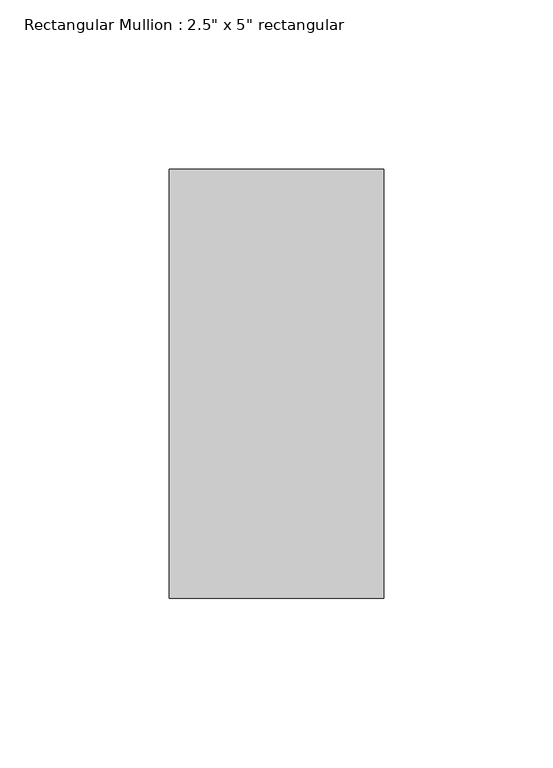
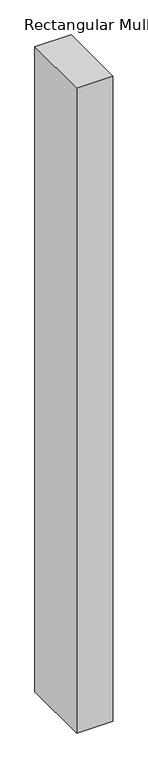
"""IFC4 building model written with IfcOpenShell, lengths in millimetres: member geometry."""

from ifc_helpers import new_model, si_unit, frame, origin, place, context, project, spatial, polyline, outline, extrude, source, transform, mapped, element, save


def member_c6549b41(model_context):
    return source(origin(), model_context, "Body", "SweptSolid", [
        extrude(outline(polyline([(31.75, 63.5), (31.75, -63.5), (-31.75, -63.5), (-31.75, 63.5), (31.75, 63.5)])), frame((0.0, 0.0, -1195.0700002), z_axis=(0.0, 0.0, 1.0), x_axis=(1.0, 0.0, 0.0)), (0.0, 0.0, 1.0), 1195.0700002),
    ])


if __name__ == "__main__":
    model = new_model("IFC4")
    model_context = context("Model", 3, world=origin())
    ifc_project = project(units=[si_unit("LENGTHUNIT", "METRE", prefix="MILLI")], contexts=[model_context])
    site = spatial("IfcSite", under=ifc_project)
    building = spatial("IfcBuilding", under=site)
    placement = place(None, origin())
    member_shape = member_c6549b41(model_context)
    element("IfcMember", 1, ObjectType="Rectangular Mullion : 2.5\" x 5\" rectangular", at=placement, inside=building, context=model_context, shape_type="MappedRepresentation", body=[
        mapped(member_shape, transform((0.0, 0.0, 0.0), x_axis=(1.0, 0.0, 0.0), y_axis=(0.0, 1.0, 0.0), z_axis=(0.0, 0.0, 1.0))),
    ])
    save(model, "model.ifc")

# Revit data of these elements
# Type "Rectangular Mullion : 2.5\" x 5\" rectangular"
#   built-in parameter 1007304 = 0.416667 (stored number, unit not read)
#   built-in parameter 1007301 = 0.104167 (stored number, unit not read)
#   built-in parameter 1007300 = 0.104167 (stored number, unit not read)
# Element 1 (IfcMember, "Rectangular Mullion : 2.5\" x 5\" rectangular")
#   Materials on its faces: "BLACK COLOUR"
# Materials
#   "BLACK COLOUR": class "Generic", colour RGB 120 120 120, transparency 0, Cost = 0
